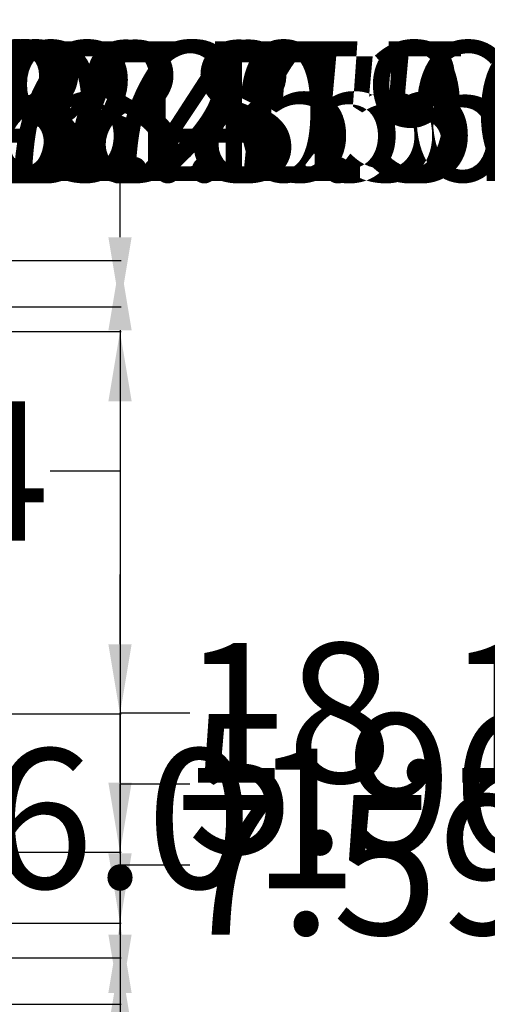
# Model space of a CAD drawing. Units: inches. Extents: x 172 to 828, y 190 to 777.
# Tile 8 of 9: x 628 to 708, y 607 to 777. Entities that reach past the tile are written whole.
import ezdxf

# ---------------------------------------------------------------- set-up
doc = ezdxf.new("R2010")
doc.units = ezdxf.units.IN
doc.header["$MEASUREMENT"] = 0
doc.layers.add('A-ANNO-DIMS', color=2, linetype='Continuous', lineweight=18)
doc.styles.get("Standard").update_dxf_attribs({"font": 'arial.ttf'})
doc.dimstyles.get("Standard").update_dxf_attribs({"dimtxt": 24, "dimasz": 12, "dimexe": 0.18, "dimexo": 0.0625, "dimgap": 0.09, "dimtad": 0, "dimtih": 1, "dimtoh": 1, "dimdec": 0, "dimzin": 0, "dimdsep": 46, "dimlunit": 3, "dimtxsty": 'Standard', "dimcen": 0.09, "dimadec": 0, "dimazin": 0, "dimtfac": 1, "dimtdec": 0, "dimtofl": 0, "dimtmove": 0, "dimatfit": 3, "dimfxl": 1, "dimtolj": 1, "dimtzin": 0, "dimarcsym": 0})

# ---------------------------------------------------------------- blocks, each defined once
blk = doc.blocks.new('*D6')
at = {"layer": 'A-ANNO-DIMS', "color": 0, "lineweight": -2, "transparency": 16777216}
for p, q in [((411.3, 579.39), (424.02, 579.39)), ((423.84, 567.39), (423.84, 549.9)), ((423.84, 507.39), (423.84, 524.88)), ((411.3, 495.39), (424.02, 495.39))]:
    blk.add_line(p, q, dxfattribs=at)
at = {"layer": 'A-ANNO-DIMS', "color": 0, "transparency": 16777216}
for points in [[(421.84, 567.39), (425.84, 567.39), (423.84, 579.39)], [(421.84, 507.39), (425.84, 507.39), (423.84, 495.39)]]:
    blk.add_solid(points, dxfattribs=at)
at = {"layer": 'Defpoints', "color": 0, "transparency": 16777216}
for p in [(411.24, 579.39), (423.84, 579.39), (411.24, 495.39)]:
    blk.add_point(p, dxfattribs=at)
at = {"layer": 'A-ANNO-DIMS', "color": 0, "transparency": 16777216, "insert": (423.84, 537.39), "char_height": 24, "attachment_point": 5}
blk.add_mtext('\\A1;GLAZED DOUBLE DOOR 84 TYP.', dxfattribs=at)
blk = doc.blocks.new('*D11')
at = {"layer": 'A-ANNO-DIMS', "color": 0, "lineweight": -2, "transparency": 16777216}
for p, q in [((618.84, 735.39), (645.16, 735.39)), ((644.98, 723.39), (644.98, 495.74)), ((644.98, 243.39), (644.98, 471.05)), ((618.84, 231.39), (645.16, 231.39))]:
    blk.add_line(p, q, dxfattribs=at)
at = {"layer": 'A-ANNO-DIMS', "color": 0, "transparency": 16777216}
for points in [[(642.98, 723.39), (646.98, 723.39), (644.98, 735.39)], [(642.98, 243.39), (646.98, 243.39), (644.98, 231.39)]]:
    blk.add_solid(points, dxfattribs=at)
at = {"layer": 'Defpoints', "color": 0, "transparency": 16777216}
for p in [(618.78, 735.39), (644.98, 735.39), (618.78, 231.39)]:
    blk.add_point(p, dxfattribs=at)
at = {"layer": 'A-ANNO-DIMS', "color": 0, "transparency": 16777216, "insert": (644.98, 483.39), "char_height": 24, "attachment_point": 5}
blk.add_mtext('\\A1;504', dxfattribs=at)
blk = doc.blocks.new('*D48')
at = {"layer": 'A-ANNO-DIMS', "color": 0, "lineweight": -2, "transparency": 16777216}
for p, q in [((512.55, 761.09), (500.55, 761.09)), ((524.55, 723.23), (524.55, 761.27)), ((532.56, 723.23), (532.56, 761.27)), ((544.56, 761.09), (556.56, 761.09))]:
    blk.add_line(p, q, dxfattribs=at)
at = {"layer": 'A-ANNO-DIMS', "color": 0, "transparency": 16777216}
for points in [[(512.55, 763.09), (512.55, 759.09), (524.55, 761.09)], [(544.56, 763.09), (544.56, 759.09), (532.56, 761.09)]]:
    blk.add_solid(points, dxfattribs=at)
at = {"layer": 'Defpoints', "color": 0, "transparency": 16777216}
for p in [(532.56, 761.09), (524.55, 723.17), (532.56, 723.17)]:
    blk.add_point(p, dxfattribs=at)
at = {"layer": 'A-ANNO-DIMS', "color": 0, "transparency": 16777216, "insert": (597.16, 761.09), "char_height": 24, "attachment_point": 5}
blk.add_mtext('\\A1;8.013', dxfattribs=at)
blk = doc.blocks.new('*D50')
at = {"layer": 'A-ANNO-DIMS', "color": 0, "lineweight": -2, "transparency": 16777216}
for p, q in [((589.47, 761.09), (577.47, 761.09)), ((601.47, 723.23), (601.47, 761.27)), ((618.78, 735.45), (618.78, 761.27)), ((630.78, 761.09), (642.78, 761.09))]:
    blk.add_line(p, q, dxfattribs=at)
at = {"layer": 'A-ANNO-DIMS', "color": 0, "transparency": 16777216}
for points in [[(589.47, 763.09), (589.47, 759.09), (601.47, 761.09)], [(630.78, 763.09), (630.78, 759.09), (618.78, 761.09)]]:
    blk.add_solid(points, dxfattribs=at)
at = {"layer": 'Defpoints', "color": 0, "transparency": 16777216}
for p in [(618.78, 761.09), (618.78, 735.39), (601.47, 723.17)]:
    blk.add_point(p, dxfattribs=at)
at = {"layer": 'A-ANNO-DIMS', "color": 0, "transparency": 16777216, "insert": (691.51, 761.09), "char_height": 24, "attachment_point": 5}
blk.add_mtext('\\A1;17.314', dxfattribs=at)
blk = doc.blocks.new('*D51')
at = {"layer": 'A-ANNO-DIMS', "color": 0, "lineweight": -2, "transparency": 16777216}
for p, q in [((644.98, 739.4), (644.98, 751.4)), ((497.2, 727.4), (645.16, 727.4)), ((601.53, 723.17), (645.16, 723.17)), ((644.98, 711.17), (644.98, 699.17)), ((644.98, 699.17), (632.98, 699.17))]:
    blk.add_line(p, q, dxfattribs=at)
at = {"layer": 'A-ANNO-DIMS', "color": 0, "transparency": 16777216}
for points in [[(642.98, 739.4), (646.98, 739.4), (644.98, 727.4)], [(642.98, 711.17), (646.98, 711.17), (644.98, 723.17)]]:
    blk.add_solid(points, dxfattribs=at)
at = {"layer": 'Defpoints', "color": 0, "transparency": 16777216}
for p in [(497.14, 727.4), (601.47, 723.17), (644.98, 723.17)]:
    blk.add_point(p, dxfattribs=at)
at = {"layer": 'A-ANNO-DIMS', "color": 0, "transparency": 16777216, "insert": (591.96, 699.17), "char_height": 24, "attachment_point": 5}
blk.add_mtext('\\A1;4.234', dxfattribs=at)
blk = doc.blocks.new('*D57')
at = {"layer": 'A-ANNO-DIMS', "color": 0, "lineweight": -2, "transparency": 16777216}
for p, q in [((515.09, 761.09), (503.09, 761.09)), ((527.09, 657.43), (527.09, 761.27)), ((533.17, 657.43), (533.17, 761.27)), ((545.17, 761.09), (557.17, 761.09))]:
    blk.add_line(p, q, dxfattribs=at)
at = {"layer": 'A-ANNO-DIMS', "color": 0, "transparency": 16777216}
for points in [[(515.09, 763.09), (515.09, 759.09), (527.09, 761.09)], [(545.17, 763.09), (545.17, 759.09), (533.17, 761.09)]]:
    blk.add_solid(points, dxfattribs=at)
at = {"layer": 'Defpoints', "color": 0, "transparency": 16777216}
for p in [(533.17, 761.09), (527.09, 657.37), (533.17, 657.37)]:
    blk.add_point(p, dxfattribs=at)
at = {"layer": 'A-ANNO-DIMS', "color": 0, "transparency": 16777216, "insert": (597.85, 761.09), "char_height": 24, "attachment_point": 5}
blk.add_mtext('\\A1;6.078', dxfattribs=at)
blk = doc.blocks.new('*D58')
at = {"layer": 'A-ANNO-DIMS', "color": 0, "lineweight": -2, "transparency": 16777216}
for p, q in [((521.17, 761.09), (509.17, 761.09)), ((533.17, 657.43), (533.17, 761.27)), ((544.89, 657.43), (544.89, 761.27)), ((556.89, 761.09), (568.89, 761.09))]:
    blk.add_line(p, q, dxfattribs=at)
at = {"layer": 'A-ANNO-DIMS', "color": 0, "transparency": 16777216}
for points in [[(521.17, 763.09), (521.17, 759.09), (533.17, 761.09)], [(556.89, 763.09), (556.89, 759.09), (544.89, 761.09)]]:
    blk.add_solid(points, dxfattribs=at)
at = {"layer": 'Defpoints', "color": 0, "transparency": 16777216}
for p in [(544.89, 761.09), (533.17, 657.37), (544.89, 657.37)]:
    blk.add_point(p, dxfattribs=at)
at = {"layer": 'A-ANNO-DIMS', "color": 0, "transparency": 16777216, "insert": (608.22, 761.09), "char_height": 24, "attachment_point": 5}
blk.add_mtext('\\A1;11.72', dxfattribs=at)
blk = doc.blocks.new('*D59')
at = {"layer": 'A-ANNO-DIMS', "color": 0, "lineweight": -2, "transparency": 16777216}
for p, q in [((532.89, 761.09), (520.89, 761.09)), ((544.89, 657.43), (544.89, 761.27)), ((550.97, 657.43), (550.97, 761.27)), ((562.97, 761.09), (574.97, 761.09))]:
    blk.add_line(p, q, dxfattribs=at)
at = {"layer": 'A-ANNO-DIMS', "color": 0, "transparency": 16777216}
for points in [[(532.89, 763.09), (532.89, 759.09), (544.89, 761.09)], [(562.97, 763.09), (562.97, 759.09), (550.97, 761.09)]]:
    blk.add_solid(points, dxfattribs=at)
at = {"layer": 'Defpoints', "color": 0, "transparency": 16777216}
for p in [(550.97, 761.09), (544.89, 657.37), (550.97, 657.37)]:
    blk.add_point(p, dxfattribs=at)
at = {"layer": 'A-ANNO-DIMS', "color": 0, "transparency": 16777216, "insert": (615.64, 761.09), "char_height": 24, "attachment_point": 5}
blk.add_mtext('\\A1;6.078', dxfattribs=at)
blk = doc.blocks.new('*D60')
at = {"layer": 'A-ANNO-DIMS', "color": 0, "lineweight": -2, "transparency": 16777216}
for p, q in [((538.97, 761.09), (526.97, 761.09)), ((550.97, 657.43), (550.97, 761.27)), ((562.69, 657.43), (562.69, 761.27)), ((574.69, 761.09), (586.69, 761.09))]:
    blk.add_line(p, q, dxfattribs=at)
at = {"layer": 'A-ANNO-DIMS', "color": 0, "transparency": 16777216}
for points in [[(538.97, 763.09), (538.97, 759.09), (550.97, 761.09)], [(574.69, 763.09), (574.69, 759.09), (562.69, 761.09)]]:
    blk.add_solid(points, dxfattribs=at)
at = {"layer": 'Defpoints', "color": 0, "transparency": 16777216}
for p in [(562.69, 761.09), (550.97, 657.37), (562.69, 657.37)]:
    blk.add_point(p, dxfattribs=at)
at = {"layer": 'A-ANNO-DIMS', "color": 0, "transparency": 16777216, "insert": (626.02, 761.09), "char_height": 24, "attachment_point": 5}
blk.add_mtext('\\A1;11.72', dxfattribs=at)
blk = doc.blocks.new('*D61')
at = {"layer": 'A-ANNO-DIMS', "color": 0, "lineweight": -2, "transparency": 16777216}
for p, q in [((550.69, 761.09), (538.69, 761.09)), ((562.69, 657.43), (562.69, 761.27)), ((568.77, 657.43), (568.77, 761.27)), ((580.77, 761.09), (592.77, 761.09))]:
    blk.add_line(p, q, dxfattribs=at)
at = {"layer": 'A-ANNO-DIMS', "color": 0, "transparency": 16777216}
for points in [[(550.69, 763.09), (550.69, 759.09), (562.69, 761.09)], [(580.77, 763.09), (580.77, 759.09), (568.77, 761.09)]]:
    blk.add_solid(points, dxfattribs=at)
at = {"layer": 'Defpoints', "color": 0, "transparency": 16777216}
for p in [(568.77, 761.09), (562.69, 657.37), (568.77, 657.37)]:
    blk.add_point(p, dxfattribs=at)
at = {"layer": 'A-ANNO-DIMS', "color": 0, "transparency": 16777216, "insert": (633.44, 761.09), "char_height": 24, "attachment_point": 5}
blk.add_mtext('\\A1;6.078', dxfattribs=at)
blk = doc.blocks.new('*D62')
at = {"layer": 'A-ANNO-DIMS', "color": 0, "lineweight": -2, "transparency": 16777216}
for p, q in [((568.77, 657.43), (568.77, 761.27)), ((580.77, 761.09), (594.82, 761.09)), ((606.82, 663.45), (606.82, 761.27)), ((606.82, 761.09), (618.82, 761.09))]:
    blk.add_line(p, q, dxfattribs=at)
at = {"layer": 'A-ANNO-DIMS', "color": 0, "transparency": 16777216}
for points in [[(580.77, 763.09), (580.77, 759.09), (568.77, 761.09)], [(594.82, 763.09), (594.82, 759.09), (606.82, 761.09)]]:
    blk.add_solid(points, dxfattribs=at)
at = {"layer": 'Defpoints', "color": 0, "transparency": 16777216}
for p in [(606.82, 761.09), (606.82, 663.39), (568.77, 657.37)]:
    blk.add_point(p, dxfattribs=at)
at = {"layer": 'A-ANNO-DIMS', "color": 0, "transparency": 16777216, "insert": (659.48, 761.09), "char_height": 24, "attachment_point": 5}
blk.add_mtext('\\A1;38.05', dxfattribs=at)
blk = doc.blocks.new('*D63')
at = {"layer": 'A-ANNO-DIMS', "color": 0, "lineweight": -2, "transparency": 16777216}
for p, q in [((594.82, 761.09), (582.82, 761.09)), ((606.82, 663.45), (606.82, 761.27)), ((618.78, 723.23), (618.78, 761.27)), ((630.78, 761.09), (642.78, 761.09))]:
    blk.add_line(p, q, dxfattribs=at)
at = {"layer": 'A-ANNO-DIMS', "color": 0, "transparency": 16777216}
for points in [[(594.82, 763.09), (594.82, 759.09), (606.82, 761.09)], [(630.78, 763.09), (630.78, 759.09), (618.78, 761.09)]]:
    blk.add_solid(points, dxfattribs=at)
at = {"layer": 'Defpoints', "color": 0, "transparency": 16777216}
for p in [(618.78, 761.09), (618.78, 723.17), (606.82, 663.39)]:
    blk.add_point(p, dxfattribs=at)
at = {"layer": 'A-ANNO-DIMS', "color": 0, "transparency": 16777216, "insert": (691.56, 761.09), "char_height": 24, "attachment_point": 5}
blk.add_mtext('\\A1;11.963', dxfattribs=at)
blk = doc.blocks.new('*D64')
at = {"layer": 'A-ANNO-DIMS', "color": 0, "lineweight": -2, "transparency": 16777216}
for p, q in [((644.98, 645.55), (644.98, 657.55)), ((644.98, 657.55), (656.98, 657.55)), ((518.47, 633.55), (645.16, 633.55)), ((518.47, 615.39), (645.16, 615.39)), ((644.98, 603.39), (644.98, 591.39))]:
    blk.add_line(p, q, dxfattribs=at)
at = {"layer": 'A-ANNO-DIMS', "color": 0, "transparency": 16777216}
for points in [[(642.98, 645.55), (646.98, 645.55), (644.98, 633.55)], [(642.98, 603.39), (646.98, 603.39), (644.98, 615.39)]]:
    blk.add_solid(points, dxfattribs=at)
at = {"layer": 'Defpoints', "color": 0, "transparency": 16777216}
for p in [(518.4, 633.55), (644.98, 633.55), (518.4, 615.39)]:
    blk.add_point(p, dxfattribs=at)
at = {"layer": 'A-ANNO-DIMS', "color": 0, "transparency": 16777216, "insert": (696.43, 657.55), "char_height": 24, "attachment_point": 5}
blk.add_mtext('\\A1;18.16', dxfattribs=at)
blk = doc.blocks.new('*D65')
at = {"layer": 'A-ANNO-DIMS', "color": 0, "lineweight": -2, "transparency": 16777216}
for p, q in [((644.98, 633.36), (644.98, 645.36)), ((644.98, 645.36), (656.98, 645.36)), ((527.16, 621.36), (645.16, 621.36)), ((518.47, 615.39), (645.16, 615.39)), ((644.98, 603.39), (644.98, 591.39))]:
    blk.add_line(p, q, dxfattribs=at)
at = {"layer": 'A-ANNO-DIMS', "color": 0, "transparency": 16777216}
for points in [[(642.98, 633.36), (646.98, 633.36), (644.98, 621.36)], [(642.98, 603.39), (646.98, 603.39), (644.98, 615.39)]]:
    blk.add_solid(points, dxfattribs=at)
at = {"layer": 'Defpoints', "color": 0, "transparency": 16777216}
for p in [(527.09, 621.36), (644.98, 621.36), (518.4, 615.39)]:
    blk.add_point(p, dxfattribs=at)
at = {"layer": 'A-ANNO-DIMS', "color": 0, "transparency": 16777216, "insert": (697.55, 645.36), "char_height": 24, "attachment_point": 5}
blk.add_mtext('\\A1;5.966', dxfattribs=at)
blk = doc.blocks.new('*D66')
at = {"layer": 'A-ANNO-DIMS', "color": 0, "lineweight": -2, "transparency": 16777216}
for p, q in [((644.98, 669.37), (644.98, 681.37)), ((568.83, 657.37), (645.16, 657.37)), ((568.83, 621.36), (645.16, 621.36)), ((644.98, 609.36), (644.98, 597.36))]:
    blk.add_line(p, q, dxfattribs=at)
at = {"layer": 'A-ANNO-DIMS', "color": 0, "transparency": 16777216}
for points in [[(642.98, 669.37), (646.98, 669.37), (644.98, 657.37)], [(642.98, 609.36), (646.98, 609.36), (644.98, 621.36)]]:
    blk.add_solid(points, dxfattribs=at)
at = {"layer": 'Defpoints', "color": 0, "transparency": 16777216}
for p in [(568.77, 657.37), (644.98, 657.37), (568.77, 621.36)]:
    blk.add_point(p, dxfattribs=at)
at = {"layer": 'A-ANNO-DIMS', "color": 0, "transparency": 16777216, "insert": (644.98, 639.36), "char_height": 24, "attachment_point": 5}
blk.add_mtext('\\A1;36.01', dxfattribs=at)
blk = doc.blocks.new('*D80')
at = {"layer": 'A-ANNO-DIMS', "color": 0, "lineweight": -2, "transparency": 16777216}
for p, q in [((487.69, 761.09), (475.69, 761.09)), ((499.69, 607.45), (499.69, 761.27)), ((517.23, 607.45), (517.23, 761.27)), ((529.23, 761.09), (541.23, 761.09))]:
    blk.add_line(p, q, dxfattribs=at)
at = {"layer": 'A-ANNO-DIMS', "color": 0, "transparency": 16777216}
for points in [[(487.69, 763.09), (487.69, 759.09), (499.69, 761.09)], [(529.23, 763.09), (529.23, 759.09), (517.23, 761.09)]]:
    blk.add_solid(points, dxfattribs=at)
at = {"layer": 'Defpoints', "color": 0, "transparency": 16777216}
for p in [(517.23, 761.09), (499.69, 607.39), (517.23, 607.39)]:
    blk.add_point(p, dxfattribs=at)
at = {"layer": 'A-ANNO-DIMS', "color": 0, "transparency": 16777216, "insert": (590, 761.09), "char_height": 24, "attachment_point": 5}
blk.add_mtext('\\A1;17.533', dxfattribs=at)
blk = doc.blocks.new('*D82')
at = {"layer": 'A-ANNO-DIMS', "color": 0, "lineweight": -2, "transparency": 16777216}
for p, q in [((588.96, 761.09), (576.96, 761.09)), ((600.96, 493.45), (600.96, 761.27)), ((606.82, 607.45), (606.82, 761.27)), ((618.82, 761.09), (630.82, 761.09))]:
    blk.add_line(p, q, dxfattribs=at)
at = {"layer": 'A-ANNO-DIMS', "color": 0, "transparency": 16777216}
for points in [[(588.96, 763.09), (588.96, 759.09), (600.96, 761.09)], [(618.82, 763.09), (618.82, 759.09), (606.82, 761.09)]]:
    blk.add_solid(points, dxfattribs=at)
at = {"layer": 'Defpoints', "color": 0, "transparency": 16777216}
for p in [(606.82, 761.09), (606.82, 607.39), (600.96, 493.39)]:
    blk.add_point(p, dxfattribs=at)
at = {"layer": 'A-ANNO-DIMS', "color": 0, "transparency": 16777216, "insert": (671.39, 761.09), "char_height": 24, "attachment_point": 5}
blk.add_mtext('\\A1;5.856', dxfattribs=at)
blk = doc.blocks.new('*D83')
at = {"layer": 'A-ANNO-DIMS', "color": 0, "lineweight": -2, "transparency": 16777216}
for p, q in [((512.83, 761.09), (500.83, 761.09)), ((524.83, 535.45), (524.83, 761.27)), ((543.3, 599.86), (543.3, 761.27)), ((555.3, 761.09), (567.3, 761.09))]:
    blk.add_line(p, q, dxfattribs=at)
at = {"layer": 'A-ANNO-DIMS', "color": 0, "transparency": 16777216}
for points in [[(512.83, 763.09), (512.83, 759.09), (524.83, 761.09)], [(555.3, 763.09), (555.3, 759.09), (543.3, 761.09)]]:
    blk.add_solid(points, dxfattribs=at)
at = {"layer": 'Defpoints', "color": 0, "transparency": 16777216}
for p in [(543.3, 761.09), (543.3, 599.8), (524.83, 535.39)]:
    blk.add_point(p, dxfattribs=at)
at = {"layer": 'A-ANNO-DIMS', "color": 0, "transparency": 16777216, "insert": (606.75, 761.09), "char_height": 24, "attachment_point": 5}
blk.add_mtext('\\A1;18.47', dxfattribs=at)
blk = doc.blocks.new('*D84')
at = {"layer": 'A-ANNO-DIMS', "color": 0, "lineweight": -2, "transparency": 16777216}
for p, q in [((543.3, 599.86), (543.3, 761.27)), ((555.3, 761.09), (579.54, 761.09)), ((591.54, 599.86), (591.54, 761.27)), ((591.54, 761.09), (603.54, 761.09))]:
    blk.add_line(p, q, dxfattribs=at)
at = {"layer": 'A-ANNO-DIMS', "color": 0, "transparency": 16777216}
for points in [[(555.3, 763.09), (555.3, 759.09), (543.3, 761.09)], [(579.54, 763.09), (579.54, 759.09), (591.54, 761.09)]]:
    blk.add_solid(points, dxfattribs=at)
at = {"layer": 'Defpoints', "color": 0, "transparency": 16777216}
for p in [(591.54, 761.09), (543.3, 599.8), (591.54, 599.8)]:
    blk.add_point(p, dxfattribs=at)
at = {"layer": 'A-ANNO-DIMS', "color": 0, "transparency": 16777216, "insert": (644.7, 761.09), "char_height": 24, "attachment_point": 5}
blk.add_mtext('\\A1;48.25', dxfattribs=at)
blk = doc.blocks.new('*D85')
at = {"layer": 'A-ANNO-DIMS', "color": 0, "lineweight": -2, "transparency": 16777216}
for p, q in [((579.54, 761.09), (567.54, 761.09)), ((591.54, 599.86), (591.54, 761.27)), ((600.96, 535.45), (600.96, 761.27)), ((612.96, 761.09), (624.96, 761.09))]:
    blk.add_line(p, q, dxfattribs=at)
at = {"layer": 'A-ANNO-DIMS', "color": 0, "transparency": 16777216}
for points in [[(579.54, 763.09), (579.54, 759.09), (591.54, 761.09)], [(612.96, 763.09), (612.96, 759.09), (600.96, 761.09)]]:
    blk.add_solid(points, dxfattribs=at)
at = {"layer": 'Defpoints', "color": 0, "transparency": 16777216}
for p in [(600.96, 761.09), (591.54, 599.8), (600.96, 535.39)]:
    blk.add_point(p, dxfattribs=at)
at = {"layer": 'A-ANNO-DIMS', "color": 0, "transparency": 16777216, "insert": (665.63, 761.09), "char_height": 24, "attachment_point": 5}
blk.add_mtext('\\A1;9.415', dxfattribs=at)
blk = doc.blocks.new('*D86')
at = {"layer": 'A-ANNO-DIMS', "color": 0, "lineweight": -2, "transparency": 16777216}
for p, q in [((512.83, 761.09), (500.83, 761.09)), ((524.83, 493.45), (524.83, 761.27)), ((530.68, 493.45), (530.68, 761.27)), ((542.68, 761.09), (554.68, 761.09))]:
    blk.add_line(p, q, dxfattribs=at)
at = {"layer": 'A-ANNO-DIMS', "color": 0, "transparency": 16777216}
for points in [[(512.83, 763.09), (512.83, 759.09), (524.83, 761.09)], [(542.68, 763.09), (542.68, 759.09), (530.68, 761.09)]]:
    blk.add_solid(points, dxfattribs=at)
at = {"layer": 'Defpoints', "color": 0, "transparency": 16777216}
for p in [(530.68, 761.09), (524.83, 493.39), (530.68, 493.39)]:
    blk.add_point(p, dxfattribs=at)
at = {"layer": 'A-ANNO-DIMS', "color": 0, "transparency": 16777216, "insert": (595.26, 761.09), "char_height": 24, "attachment_point": 5}
blk.add_mtext('\\A1;5.856', dxfattribs=at)
blk = doc.blocks.new('*D91')
at = {"layer": 'A-ANNO-DIMS', "color": 0, "lineweight": -2, "transparency": 16777216}
for p, q in [((644.98, 619.39), (644.98, 631.39)), ((644.98, 631.39), (656.98, 631.39)), ((606.88, 607.39), (645.16, 607.39)), ((591.61, 599.8), (645.16, 599.8)), ((644.98, 587.8), (644.98, 575.8))]:
    blk.add_line(p, q, dxfattribs=at)
at = {"layer": 'A-ANNO-DIMS', "color": 0, "transparency": 16777216}
for points in [[(642.98, 619.39), (646.98, 619.39), (644.98, 607.39)], [(642.98, 587.8), (646.98, 587.8), (644.98, 599.8)]]:
    blk.add_solid(points, dxfattribs=at)
at = {"layer": 'Defpoints', "color": 0, "transparency": 16777216}
for p in [(606.82, 607.39), (644.98, 607.39), (591.54, 599.8)]:
    blk.add_point(p, dxfattribs=at)
at = {"layer": 'A-ANNO-DIMS', "color": 0, "transparency": 16777216, "insert": (695.15, 631.39), "char_height": 24, "attachment_point": 5}
blk.add_mtext('\\A1;7.591', dxfattribs=at)

msp = doc.modelspace()

# ---------------------------------------------------------------- dimensions: what is measured, and where the dimension line sits
at = {"layer": 'A-ANNO-DIMS'}
for base, p1, p2, override, picture, middle in [((517.2267, 761.0923), (499.6941, 607.3923), (517.2267, 607.3923), {"dimdec": 3, "dimlfac": 1, "dimrnd": 0, "dimzin": 0, "dimdsep": 46, "dimlunit": 2}, '*D80', (590.0043, 761.0923)), ((532.56368, 761.09229), (524.55022, 723.16837), (532.56368, 723.16837), {"dimdec": 3, "dimlfac": 1, "dimrnd": 0, "dimzin": 0, "dimdsep": 46, "dimlunit": 2}, '*D48', (597.16391, 761.09229)), ((543.2956, 761.0923), (524.8269, 535.3923), (543.2956, 599.8013), {"dimdec": 2, "dimlfac": 1, "dimrnd": 0, "dimzin": 0, "dimdsep": 46, "dimlunit": 2}, '*D83', (606.7498, 761.0923)), ((530.6832, 761.0923), (524.8269, 493.3923), (530.6832, 493.3923), {"dimdec": 3, "dimlfac": 1, "dimrnd": 0, "dimzin": 0, "dimdsep": 46, "dimlunit": 2}, '*D86', (595.2589, 761.0923)), ((533.1719, 761.0923), (527.0943, 657.3703), (533.1719, 657.3703), {"dimdec": 3, "dimlfac": 1, "dimrnd": 0, "dimzin": 0, "dimdsep": 46, "dimlunit": 2}, '*D57', (597.8458, 761.0923)), ((544.8929, 761.0923), (533.1719, 657.3703), (544.8929, 657.3703), {"dimdec": 2, "dimlfac": 1, "dimrnd": 0, "dimzin": 0, "dimdsep": 46, "dimlunit": 2}, '*D58', (608.2244, 761.0923)), ((550.9705, 761.0923), (544.8929, 657.3703), (550.9705, 657.3703), {"dimdec": 3, "dimlfac": 1, "dimrnd": 0, "dimzin": 0, "dimdsep": 46, "dimlunit": 2}, '*D59', (615.6444, 761.0923)), ((562.6916, 761.0923), (550.9705, 657.3703), (562.6916, 657.3703), {"dimdec": 2, "dimlfac": 1, "dimrnd": 0, "dimzin": 0, "dimdsep": 46, "dimlunit": 2}, '*D60', (626.023, 761.0923)), ((568.7692, 761.0923), (562.6916, 657.3703), (568.7692, 657.3703), {"dimdec": 3, "dimlfac": 1, "dimrnd": 0, "dimzin": 0, "dimdsep": 46, "dimlunit": 2}, '*D61', (633.4431, 761.0923)), ((591.5446, 761.0923), (543.2956, 599.8013), (591.5446, 599.8013), {"dimdec": 2, "dimlfac": 1, "dimrnd": 0, "dimzin": 0, "dimdsep": 46, "dimlunit": 2}, '*D84', (644.7014, 761.0923)), ((600.9594, 761.0923), (591.5446, 599.8013), (600.9594, 535.3923), {"dimdec": 3, "dimlfac": 1, "dimrnd": 0, "dimzin": 0, "dimdsep": 46, "dimlunit": 2}, '*D85', (665.6333, 761.0923)), ((606.8158, 761.0923), (568.7692, 657.3703), (606.8158, 663.3923), {"dimdec": 2, "dimlfac": 1, "dimrnd": 0, "dimzin": 0, "dimdsep": 46, "dimlunit": 2}, '*D62', (659.4815, 761.0923)), ((606.8158, 761.0923), (600.9594, 493.3923), (606.8158, 607.3923), {"dimdec": 3, "dimlfac": 1, "dimrnd": 0, "dimzin": 0, "dimdsep": 46, "dimlunit": 2}, '*D82', (671.3915, 761.0923)), ((618.7792, 761.0923), (601.4651, 723.1684), (618.7792, 735.3923), {"dimdec": 3, "dimlfac": 1, "dimrnd": 0, "dimzin": 0, "dimdsep": 46, "dimlunit": 2}, '*D50', (691.5076, 761.0923)), ((618.7792, 761.0923), (606.8158, 663.3923), (618.7792, 723.1684), {"dimdec": 3, "dimlfac": 1, "dimrnd": 0, "dimzin": 0, "dimdsep": 46, "dimlunit": 2}, '*D63', (691.5568, 761.0923))]:
    dim = msp.add_linear_dim(base=base, p1=p1, p2=p2, dimstyle='Standard', override=override, dxfattribs=at)
    dim.commit()
    dim.dimension.update_dxf_attribs({"geometry": picture, "text_midpoint": middle})
for base, p1, p2, override, picture, middle in [((644.9792, 723.1684), (497.1421, 727.4027), (601.4651, 723.1684), {"dimdec": 3, "dimlfac": 1, "dimrnd": 0, "dimzin": 0, "dimdsep": 46, "dimlunit": 2}, '*D51', (591.9615, 699.1684)), ((644.9792, 735.3923), (618.7792, 231.3923), (618.7792, 735.3923), {"dimdec": 0, "dimlfac": 1, "dimrnd": 0, "dimzin": 0, "dimdsep": 46, "dimlunit": 2}, '*D11', (644.9792, 483.3923)), ((644.9792, 657.3703), (568.7692, 621.358), (568.7692, 657.3703), {"dimdec": 2, "dimlfac": 1, "dimrnd": 0, "dimzin": 0, "dimdsep": 46, "dimlunit": 2}, '*D66', (644.9792, 639.3642)), ((644.9792, 633.5521), (518.4045, 615.3923), (518.4045, 633.5521), {"dimdec": 2, "dimlfac": 1, "dimrnd": 0, "dimzin": 0, "dimdsep": 46, "dimlunit": 2}, '*D64', (696.4252, 657.5521)), ((644.9792, 621.358), (518.4045, 615.3923), (527.0943, 621.358), {"dimdec": 3, "dimlfac": 1, "dimrnd": 0, "dimzin": 0, "dimdsep": 46, "dimlunit": 2}, '*D65', (697.5549, 645.358)), ((644.9792, 607.3923), (591.5446, 599.8013), (606.8158, 607.3923), {"dimdec": 3, "dimlfac": 1, "dimrnd": 0, "dimzin": 0, "dimdsep": 46, "dimlunit": 2}, '*D91', (695.1483, 631.3923))]:
    dim = msp.add_linear_dim(base=base, p1=p1, p2=p2, angle=90, dimstyle='Standard', override=override, dxfattribs=at)
    dim.commit()
    dim.dimension.update_dxf_attribs({"geometry": picture, "text_midpoint": middle})
dim = msp.add_linear_dim(base=(423.8362, 579.3923), p1=(411.2362, 495.3923), p2=(411.2362, 579.3923), angle=90, text='GLAZED DOUBLE DOOR <> TYP.', dimstyle='Standard', override={"dimdec": 0, "dimlfac": 1, "dimrnd": 0, "dimzin": 0, "dimdsep": 46, "dimlunit": 2}, dxfattribs=at)
dim.commit()
dim.dimension.update_dxf_attribs({"geometry": '*D6', "text_midpoint": (423.8362, 537.3923)})

doc.saveas('drawing.dxf')
